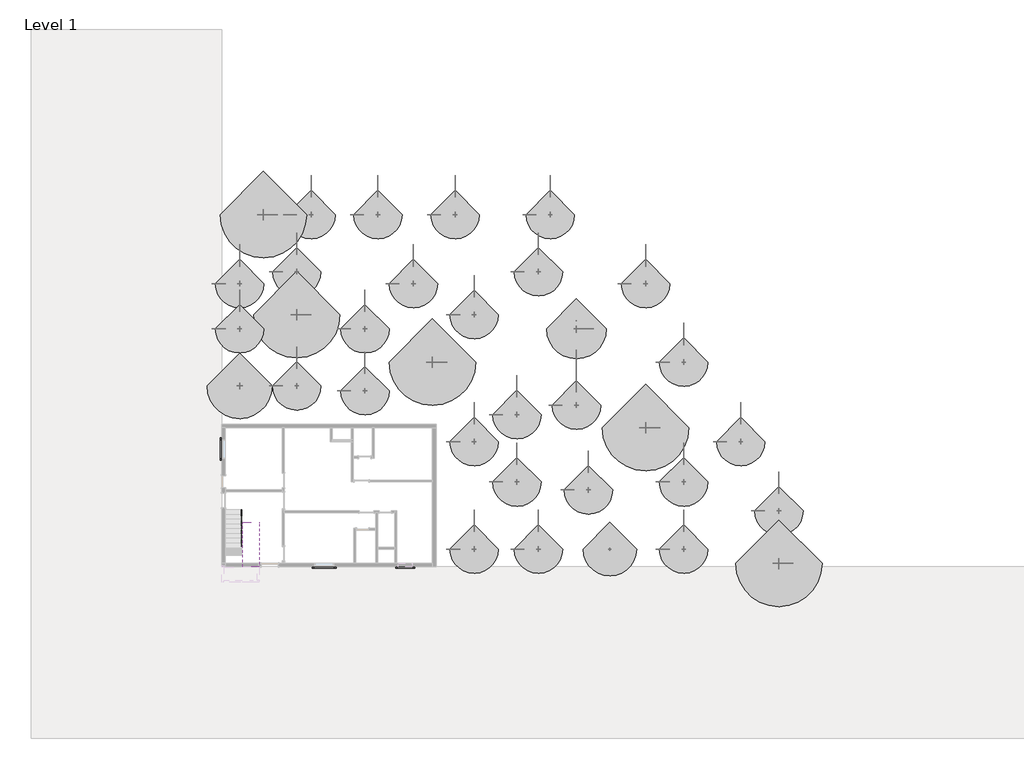
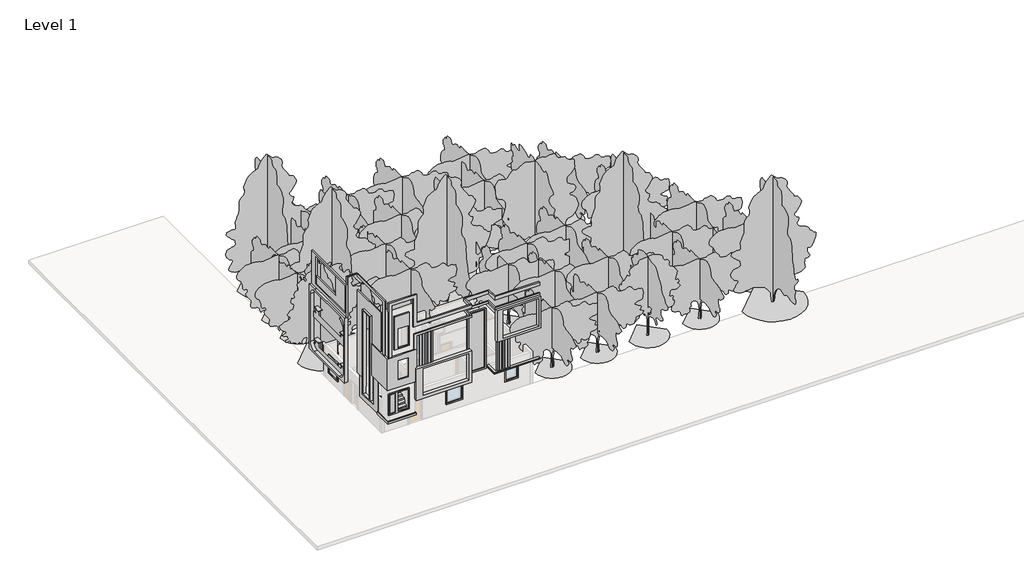
# One storey, part 2 of 2: 34 geographic elements, 1 proxy, 1 railing, 1 stair flight.
"""IFC4 building model written with IfcOpenShell, lengths in millimetres."""

from ifc_helpers import new_model, si_unit, frame, origin, place, context, project, spatial, polyline, outline, extrude, faceted_brep, transform, mapped, element, save
from components import generic_models_1_generic_models_1_784ad703, rpc_tree_deciduous_common_apple_20_2cf08d23, rpc_tree_deciduous_largetooth_aspen_25_f6cd7aa4, rpc_tree_deciduous_lombardy_poplar_40_01077960, rpc_tree_deciduous_red_maple_30_cba750cc, rpc_tree_deciduous_schumard_oak_30_cf07c7db

model = new_model("IFC4")

# Units and contexts
model_context = context("Model", 3, world=origin())
ifc_project = project(units=[si_unit("LENGTHUNIT", "METRE", prefix="MILLI")], contexts=[model_context])

# Site, building, storey
site = spatial("IfcSite", under=ifc_project)
building = spatial("IfcBuilding", under=site)
storey = spatial("IfcBuildingStorey", under=building, Name="Level 1", Elevation=0.0)

# Proxy
placement = place(None, origin())
generic_models_1_generic_models_1_shape = generic_models_1_generic_models_1_784ad703(model_context)
element("IfcBuildingElementProxy", 1, Name="Generic Models 1 : Generic Models 1", ObjectType="Generic Models 1 : Generic Models 1", at=placement, inside=storey, context=model_context, shape_type="MappedRepresentation", body=[
    mapped(generic_models_1_generic_models_1_shape, transform((0.0, 0.0, 0.0), x_axis=(1.0, 0.0, 0.0), y_axis=(0.0, 1.0, 0.0), z_axis=(0.0, 0.0, 1.0))),
])

# Geographic elements
rpc_tree_deciduous_common_apple_20_shape = rpc_tree_deciduous_common_apple_20_2cf08d23(model_context)
element("IfcGeographicElement", 2, ObjectType="RPC Tree - Deciduous : Common Apple - 20'", at=placement, inside=storey, context=model_context, shape_type="MappedRepresentation", body=[
    mapped(rpc_tree_deciduous_common_apple_20_shape, transform((-9198.7394758, 21766.0495492, 0.0), x_axis=(1.0, 0.0, 0.0), y_axis=(0.0, 1.0, 0.0), z_axis=(0.0, 0.0, 1.0))),
])
element("IfcGeographicElement", 3, ObjectType="RPC Tree - Deciduous : Common Apple - 20'", at=placement, inside=storey, context=model_context, shape_type="MappedRepresentation", body=[
    mapped(rpc_tree_deciduous_common_apple_20_shape, transform((-9198.7394758, 18870.4495492, 0.0), x_axis=(1.0, 0.0, 0.0), y_axis=(0.0, 1.0, 0.0), z_axis=(0.0, 0.0, 1.0))),
])
element("IfcGeographicElement", 4, ObjectType="RPC Tree - Deciduous : Common Apple - 20'", at=placement, inside=storey, context=model_context, shape_type="MappedRepresentation", body=[
    mapped(rpc_tree_deciduous_common_apple_20_shape, transform((-5541.1394758, 15212.8495492, 0.0), x_axis=(1.0, 0.0, 0.0), y_axis=(0.0, 1.0, 0.0), z_axis=(0.0, 0.0, 1.0))),
])
element("IfcGeographicElement", 5, ObjectType="RPC Tree - Deciduous : Common Apple - 20'", at=placement, inside=storey, context=model_context, shape_type="MappedRepresentation", body=[
    mapped(rpc_tree_deciduous_common_apple_20_shape, transform((-1172.3394758, 18870.4495492, 0.0), x_axis=(1.0, 0.0, 0.0), y_axis=(0.0, 1.0, 0.0), z_axis=(0.0, 0.0, 1.0))),
])
element("IfcGeographicElement", 6, ObjectType="RPC Tree - Deciduous : Common Apple - 20'", at=placement, inside=storey, context=model_context, shape_type="MappedRepresentation", body=[
    mapped(rpc_tree_deciduous_common_apple_20_shape, transform((-1172.3394758, 14908.0495492, 0.0), x_axis=(1.0, 0.0, 0.0), y_axis=(0.0, 1.0, 0.0), z_axis=(0.0, 0.0, 1.0))),
])
element("IfcGeographicElement", 7, ObjectType="RPC Tree - Deciduous : Common Apple - 20'", at=placement, inside=storey, context=model_context, shape_type="MappedRepresentation", body=[
    mapped(rpc_tree_deciduous_common_apple_20_shape, transform((5812.6605242, 4773.4495492, 0.0), x_axis=(1.0, 0.0, 0.0), y_axis=(0.0, 1.0, 0.0), z_axis=(0.0, 0.0, 1.0))),
])
element("IfcGeographicElement", 8, ObjectType="RPC Tree - Deciduous : Common Apple - 20'", at=placement, inside=storey, context=model_context, shape_type="MappedRepresentation", body=[
    mapped(rpc_tree_deciduous_common_apple_20_shape, transform((9927.4605242, 4773.4495492, 0.0), x_axis=(1.0, 0.0, 0.0), y_axis=(0.0, 1.0, 0.0), z_axis=(0.0, 0.0, 1.0))),
])
element("IfcGeographicElement", 9, ObjectType="RPC Tree - Deciduous : Common Apple - 20'", at=placement, inside=storey, context=model_context, shape_type="MappedRepresentation", body=[
    mapped(rpc_tree_deciduous_common_apple_20_shape, transform((13127.8605242, 8558.0495492, 0.0), x_axis=(1.0, 0.0, 0.0), y_axis=(0.0, 1.0, 0.0), z_axis=(0.0, 0.0, 1.0))),
])
element("IfcGeographicElement", 10, ObjectType="RPC Tree - Deciduous : Common Apple - 20'", at=placement, inside=storey, context=model_context, shape_type="MappedRepresentation", body=[
    mapped(rpc_tree_deciduous_common_apple_20_shape, transform((8555.8605242, 9066.0495492, 0.0), x_axis=(1.0, 0.0, 0.0), y_axis=(0.0, 1.0, 0.0), z_axis=(0.0, 0.0, 1.0))),
])
element("IfcGeographicElement", 11, ObjectType="RPC Tree - Deciduous : Common Apple - 20'", at=placement, inside=storey, context=model_context, shape_type="MappedRepresentation", body=[
    mapped(rpc_tree_deciduous_common_apple_20_shape, transform((8555.8605242, 13384.0495492, 0.0), x_axis=(1.0, 0.0, 0.0), y_axis=(0.0, 1.0, 0.0), z_axis=(0.0, 0.0, 1.0))),
])
element("IfcGeographicElement", 12, ObjectType="RPC Tree - Deciduous : Common Apple - 20'", at=placement, inside=storey, context=model_context, shape_type="MappedRepresentation", body=[
    mapped(rpc_tree_deciduous_common_apple_20_shape, transform((12365.8605242, 13993.6495492, 0.0), x_axis=(1.0, 0.0, 0.0), y_axis=(0.0, 1.0, 0.0), z_axis=(0.0, 0.0, 1.0))),
])
element("IfcGeographicElement", 13, ObjectType="RPC Tree - Deciduous : Common Apple - 20'", at=placement, inside=storey, context=model_context, shape_type="MappedRepresentation", body=[
    mapped(rpc_tree_deciduous_common_apple_20_shape, transform((5812.6605242, 11656.8495492, 0.0), x_axis=(1.0, 0.0, 0.0), y_axis=(0.0, 1.0, 0.0), z_axis=(0.0, 0.0, 1.0))),
])
element("IfcGeographicElement", 14, ObjectType="RPC Tree - Deciduous : Common Apple - 20'", at=placement, inside=storey, context=model_context, shape_type="MappedRepresentation", body=[
    mapped(rpc_tree_deciduous_common_apple_20_shape, transform((19223.8605242, 4773.4495492, 0.0), x_axis=(1.0, 0.0, 0.0), y_axis=(0.0, 1.0, 0.0), z_axis=(0.0, 0.0, 1.0))),
])
element("IfcGeographicElement", 15, ObjectType="RPC Tree - Deciduous : Common Apple - 20'", at=placement, inside=storey, context=model_context, shape_type="MappedRepresentation", body=[
    mapped(rpc_tree_deciduous_common_apple_20_shape, transform((19223.8605242, 9066.0495492, 0.0), x_axis=(1.0, 0.0, 0.0), y_axis=(0.0, 1.0, 0.0), z_axis=(0.0, 0.0, 1.0))),
])
element("IfcGeographicElement", 16, ObjectType="RPC Tree - Deciduous : Common Apple - 20'", at=placement, inside=storey, context=model_context, shape_type="MappedRepresentation", body=[
    mapped(rpc_tree_deciduous_common_apple_20_shape, transform((5812.6605242, 19784.8495492, 0.0), x_axis=(1.0, 0.0, 0.0), y_axis=(0.0, 1.0, 0.0), z_axis=(0.0, 0.0, 1.0))),
])
element("IfcGeographicElement", 17, ObjectType="RPC Tree - Deciduous : Common Apple - 20'", at=placement, inside=storey, context=model_context, shape_type="MappedRepresentation", body=[
    mapped(rpc_tree_deciduous_common_apple_20_shape, transform((1926.4605242, 21766.0495492, 0.0), x_axis=(1.0, 0.0, 0.0), y_axis=(0.0, 1.0, 0.0), z_axis=(0.0, 0.0, 1.0))),
])
element("IfcGeographicElement", 18, ObjectType="RPC Tree - Deciduous : Common Apple - 20'", at=placement, inside=storey, context=model_context, shape_type="MappedRepresentation", body=[
    mapped(rpc_tree_deciduous_common_apple_20_shape, transform((9927.4605242, 22528.0495492, 0.0), x_axis=(1.0, 0.0, 0.0), y_axis=(0.0, 1.0, 0.0), z_axis=(0.0, 0.0, 1.0))),
])
element("IfcGeographicElement", 19, ObjectType="RPC Tree - Deciduous : Common Apple - 20'", at=placement, inside=storey, context=model_context, shape_type="MappedRepresentation", body=[
    mapped(rpc_tree_deciduous_common_apple_20_shape, transform((16785.4605242, 21766.0495492, 0.0), x_axis=(1.0, 0.0, 0.0), y_axis=(0.0, 1.0, 0.0), z_axis=(0.0, 0.0, 1.0))),
])
element("IfcGeographicElement", 20, ObjectType="RPC Tree - Deciduous : Common Apple - 20'", at=placement, inside=storey, context=model_context, shape_type="MappedRepresentation", body=[
    mapped(rpc_tree_deciduous_common_apple_20_shape, transform((19223.8605242, 16736.8495492, 0.0), x_axis=(1.0, 0.0, 0.0), y_axis=(0.0, 1.0, 0.0), z_axis=(0.0, 0.0, 1.0))),
])
element("IfcGeographicElement", 21, ObjectType="RPC Tree - Deciduous : Common Apple - 20'", at=placement, inside=storey, context=model_context, shape_type="MappedRepresentation", body=[
    mapped(rpc_tree_deciduous_common_apple_20_shape, transform((22881.4605242, 11656.8495492, 0.0), x_axis=(1.0, 0.0, 0.0), y_axis=(0.0, 1.0, 0.0), z_axis=(0.0, 0.0, 1.0))),
])
element("IfcGeographicElement", 22, ObjectType="RPC Tree - Deciduous : Common Apple - 20'", at=placement, inside=storey, context=model_context, shape_type="MappedRepresentation", body=[
    mapped(rpc_tree_deciduous_common_apple_20_shape, transform((25319.8605242, 7211.8495492, 0.0), x_axis=(1.0, 0.0, 0.0), y_axis=(0.0, 1.0, 0.0), z_axis=(0.0, 0.0, 1.0))),
])
element("IfcGeographicElement", 23, ObjectType="RPC Tree - Deciduous : Common Apple - 20'", at=placement, inside=storey, context=model_context, shape_type="MappedRepresentation", body=[
    mapped(rpc_tree_deciduous_common_apple_20_shape, transform((-4626.7394758, 26185.6495492, 0.0), x_axis=(1.0, 0.0, 0.0), y_axis=(0.0, 1.0, 0.0), z_axis=(0.0, 0.0, 1.0))),
])
element("IfcGeographicElement", 24, ObjectType="RPC Tree - Deciduous : Common Apple - 20'", at=placement, inside=storey, context=model_context, shape_type="MappedRepresentation", body=[
    mapped(rpc_tree_deciduous_common_apple_20_shape, transform((-346.8394758, 26185.6495492, 0.0), x_axis=(1.0, 0.0, 0.0), y_axis=(0.0, 1.0, 0.0), z_axis=(0.0, 0.0, 1.0))),
])
element("IfcGeographicElement", 25, ObjectType="RPC Tree - Deciduous : Common Apple - 20'", at=placement, inside=storey, context=model_context, shape_type="MappedRepresentation", body=[
    mapped(rpc_tree_deciduous_common_apple_20_shape, transform((-5541.1394758, 22528.0495492, 0.0), x_axis=(1.0, 0.0, 0.0), y_axis=(0.0, 1.0, 0.0), z_axis=(0.0, 0.0, 1.0))),
])
element("IfcGeographicElement", 26, ObjectType="RPC Tree - Deciduous : Common Apple - 20'", at=placement, inside=storey, context=model_context, shape_type="MappedRepresentation", body=[
    mapped(rpc_tree_deciduous_common_apple_20_shape, transform((4593.4605242, 26185.6495492, 0.0), x_axis=(1.0, 0.0, 0.0), y_axis=(0.0, 1.0, 0.0), z_axis=(0.0, 0.0, 1.0))),
])
element("IfcGeographicElement", 27, ObjectType="RPC Tree - Deciduous : Common Apple - 20'", at=placement, inside=storey, context=model_context, shape_type="MappedRepresentation", body=[
    mapped(rpc_tree_deciduous_common_apple_20_shape, transform((10689.4605242, 26185.6495492, 0.0), x_axis=(1.0, 0.0, 0.0), y_axis=(0.0, 1.0, 0.0), z_axis=(0.0, 0.0, 1.0))),
])
rpc_tree_deciduous_largetooth_aspen_25_shape = rpc_tree_deciduous_largetooth_aspen_25_f6cd7aa4(model_context)
element("IfcGeographicElement", 28, ObjectType="RPC Tree - Deciduous : Largetooth Aspen - 25'", at=placement, inside=storey, context=model_context, shape_type="MappedRepresentation", body=[
    mapped(rpc_tree_deciduous_largetooth_aspen_25_shape, transform((14499.4605242, 4773.4495492, 0.0), x_axis=(1.0, 0.0, 0.0), y_axis=(0.0, 1.0, 0.0), z_axis=(0.0, 0.0, 1.0))),
])
rpc_tree_deciduous_lombardy_poplar_40_shape = rpc_tree_deciduous_lombardy_poplar_40_01077960(model_context)
element("IfcGeographicElement", 29, ObjectType="RPC Tree - Deciduous : Lombardy Poplar - 40'", at=placement, inside=storey, context=model_context, shape_type="MappedRepresentation", body=[
    mapped(rpc_tree_deciduous_lombardy_poplar_40_shape, transform((-5541.1394758, 19784.8495492, 0.0), x_axis=(1.0, 0.0, 0.0), y_axis=(0.0, 1.0, 0.0), z_axis=(0.0, 0.0, 1.0))),
])
element("IfcGeographicElement", 30, ObjectType="RPC Tree - Deciduous : Lombardy Poplar - 40'", at=placement, inside=storey, context=model_context, shape_type="MappedRepresentation", body=[
    mapped(rpc_tree_deciduous_lombardy_poplar_40_shape, transform((3145.6605242, 16736.8495492, 0.0), x_axis=(1.0, 0.0, 0.0), y_axis=(0.0, 1.0, 0.0), z_axis=(0.0, 0.0, 1.0))),
])
element("IfcGeographicElement", 31, ObjectType="RPC Tree - Deciduous : Lombardy Poplar - 40'", at=placement, inside=storey, context=model_context, shape_type="MappedRepresentation", body=[
    mapped(rpc_tree_deciduous_lombardy_poplar_40_shape, transform((16785.4605242, 12545.8495492, 0.0), x_axis=(1.0, 0.0, 0.0), y_axis=(0.0, 1.0, 0.0), z_axis=(0.0, 0.0, 1.0))),
])
element("IfcGeographicElement", 32, ObjectType="RPC Tree - Deciduous : Lombardy Poplar - 40'", at=placement, inside=storey, context=model_context, shape_type="MappedRepresentation", body=[
    mapped(rpc_tree_deciduous_lombardy_poplar_40_shape, transform((25319.8605242, 3859.0495492, 0.0), x_axis=(1.0, 0.0, 0.0), y_axis=(0.0, 1.0, 0.0), z_axis=(0.0, 0.0, 1.0))),
])
element("IfcGeographicElement", 33, ObjectType="RPC Tree - Deciduous : Lombardy Poplar - 40'", at=placement, inside=storey, context=model_context, shape_type="MappedRepresentation", body=[
    mapped(rpc_tree_deciduous_lombardy_poplar_40_shape, transform((-7674.7394758, 26185.6495492, 0.0), x_axis=(1.0, 0.0, 0.0), y_axis=(0.0, 1.0, 0.0), z_axis=(0.0, 0.0, 1.0))),
])
rpc_tree_deciduous_red_maple_30_shape = rpc_tree_deciduous_red_maple_30_cba750cc(model_context)
element("IfcGeographicElement", 34, ObjectType="RPC Tree - Deciduous : Red Maple - 30'", at=placement, inside=storey, context=model_context, shape_type="MappedRepresentation", body=[
    mapped(rpc_tree_deciduous_red_maple_30_shape, transform((-9198.7394758, 15212.8495492, 0.0), x_axis=(1.0, 0.0, 0.0), y_axis=(0.0, 1.0, 0.0), z_axis=(0.0, 0.0, 1.0))),
])
rpc_tree_deciduous_schumard_oak_30_shape = rpc_tree_deciduous_schumard_oak_30_cf07c7db(model_context)
element("IfcGeographicElement", 35, ObjectType="RPC Tree - Deciduous : Schumard Oak - 30'", at=placement, inside=storey, context=model_context, shape_type="MappedRepresentation", body=[
    mapped(rpc_tree_deciduous_schumard_oak_30_shape, transform((12365.8605242, 18870.4495492, 0.0), x_axis=(1.0, 0.0, 0.0), y_axis=(0.0, 1.0, 0.0), z_axis=(0.0, 0.0, 1.0))),
])

# Railing
element("IfcRailing", 36, ObjectType="Handrail - Rectangular", at=placement, inside=storey, context=model_context, shape_type="SolidModel", body=[
    faceted_brep([(-9046.3394758, 7288.0495492, 1059.5428571), (-9046.3394758, 7288.0495492, 1003.2772447), (-9097.1394758, 7288.0495492, 1003.2772447), (-9097.1394758, 7288.0495492, 1059.5428571), (-9046.3394758, 3935.2495492, 2656.1142857), (-9046.3394758, 3923.7717632, 2605.3142857), (-9097.1394758, 3923.7717632, 2605.3142857), (-9097.1394758, 3935.2495492, 2656.1142857), (-9046.3394758, 3630.4495492, 2656.1142857), (-9097.1394758, 3630.4495492, 2656.1142857), (-9097.1394758, 3579.6495492, 2605.3142857), (-9046.3394758, 3579.6495492, 2605.3142857)], [[[0, 1, 2, 3]], [[1, 0, 4, 5]], [[2, 1, 5, 6]], [[3, 2, 6, 7]], [[0, 3, 7, 4]], [[8, 9, 10, 11]], [[5, 4, 8, 11]], [[6, 5, 11, 10]], [[7, 6, 10, 9]], [[4, 7, 9, 8]]]),
    faceted_brep([(-9046.3394758, 3630.4495492, 2656.1142857), (-9046.3394758, 3579.6495492, 2605.3142857), (-9097.1394758, 3579.6495492, 2605.3142857), (-9097.1394758, 3630.4495492, 2656.1142857), (-9046.3394758, 3630.4495492, 2786.7428571), (-9097.1394758, 3630.4495492, 2837.5428571), (-9097.1394758, 3579.6495492, 2837.5428571), (-9046.3394758, 3579.6495492, 2786.7428571)], [[[0, 1, 2, 3]], [[4, 5, 6, 7]], [[1, 0, 4, 7]], [[2, 1, 7, 6]], [[3, 2, 6, 5]], [[0, 3, 5, 4]]]),
    faceted_brep([(-9097.1394758, 3630.4495492, 2837.5428571), (-9046.3394758, 3630.4495492, 2786.7428571), (-9046.3394758, 3579.6495492, 2786.7428571), (-9097.1394758, 3579.6495492, 2837.5428571), (-8995.5394758, 3630.4495492, 2837.5428571), (-8995.5394758, 3630.4495492, 2786.7428571), (-8944.7394758, 3579.6495492, 2786.7428571), (-8944.7394758, 3579.6495492, 2837.5428571), (-8995.5394758, 3706.6495492, 2837.5428571), (-8995.5394758, 3718.1273353, 2786.7428571), (-8944.7394758, 3718.1273353, 2786.7428571), (-8944.7394758, 3706.6495492, 2837.5428571), (-8995.5394758, 6068.8495492, 3962.4), (-8995.5394758, 6080.3273353, 3911.6), (-8944.7394758, 6080.3273353, 3911.6), (-8944.7394758, 6068.8495492, 3962.4), (-8995.5394758, 6373.6495492, 3962.4), (-8944.7394758, 6373.6495492, 3962.4), (-8944.7394758, 6373.6495492, 3911.6), (-8995.5394758, 6373.6495492, 3911.6)], [[[0, 1, 2, 3]], [[1, 0, 4, 5]], [[2, 1, 5, 6]], [[3, 2, 6, 7]], [[0, 3, 7, 4]], [[5, 4, 8, 9]], [[6, 5, 9, 10]], [[7, 6, 10, 11]], [[4, 7, 11, 8]], [[9, 8, 12, 13]], [[10, 9, 13, 14]], [[11, 10, 14, 15]], [[8, 11, 15, 12]], [[16, 17, 18, 19]], [[13, 12, 16, 19]], [[14, 13, 19, 18]], [[15, 14, 18, 17]], [[12, 15, 17, 16]]]),
    extrude(outline(polyline([(-8979.6644758, 6338.7245492), (-8979.6644758, 6357.7745492), (-8960.6144758, 6357.7745492), (-8960.6144758, 6338.7245492), (-8979.6644758, 6338.7245492)])), frame((0.0, 0.0, 3048.0), z_axis=(0.0, 0.0, 1.0), x_axis=(1.0, 0.0, 0.0)), (0.0, 0.0, 1.0), 863.6),
    extrude(outline(polyline([(-8979.6644758, 6237.1245492), (-8979.6644758, 6256.1745492), (-8960.6144758, 6256.1745492), (-8960.6144758, 6237.1245492), (-8979.6644758, 6237.1245492)])), frame((0.0, 0.0, 3048.0), z_axis=(0.0, 0.0, 1.0), x_axis=(1.0, 0.0, 0.0)), (0.0, 0.0, 1.0), 863.6),
    extrude(outline(polyline([(-8979.6644758, 6135.5245492), (-8979.6644758, 6154.5745492), (-8960.6144758, 6154.5745492), (-8960.6144758, 6135.5245492), (-8979.6644758, 6135.5245492)])), frame((0.0, 0.0, 3048.0), z_axis=(0.0, 0.0, 1.0), x_axis=(1.0, 0.0, 0.0)), (0.0, 0.0, 1.0), 863.6),
    extrude(outline(polyline([(6052.9745492, 3898.5748638), (6052.9745492, 2902.8571429), (6033.9245492, 2902.8571429), (6033.9245492, 3889.5034352), (6052.9745492, 3898.5748638)])), frame((-8979.6644758, 0.0, 0.0), z_axis=(1.0, 0.0, 0.0), x_axis=(0.0, 1.0, 0.0)), (0.0, 0.0, 1.0), 19.05),
    extrude(outline(polyline([(5951.3745492, 3850.1939114), (5951.3745492, 2902.8571429), (5932.3245492, 2902.8571429), (5932.3245492, 3841.1224828), (5951.3745492, 3850.1939114)])), frame((-8979.6644758, 0.0, 0.0), z_axis=(1.0, 0.0, 0.0), x_axis=(0.0, 1.0, 0.0)), (0.0, 0.0, 1.0), 19.05),
    extrude(outline(polyline([(5849.7745492, 3801.812959), (5849.7745492, 2902.8571429), (5830.7245492, 2902.8571429), (5830.7245492, 3792.7415305), (5849.7745492, 3801.812959)])), frame((-8979.6644758, 0.0, 0.0), z_axis=(1.0, 0.0, 0.0), x_axis=(0.0, 1.0, 0.0)), (0.0, 0.0, 1.0), 19.05),
    extrude(outline(polyline([(5748.1745492, 3753.4320067), (5748.1745492, 2757.7142857), (5729.1245492, 2757.7142857), (5729.1245492, 3744.3605781), (5748.1745492, 3753.4320067)])), frame((-8979.6644758, 0.0, 0.0), z_axis=(1.0, 0.0, 0.0), x_axis=(0.0, 1.0, 0.0)), (0.0, 0.0, 1.0), 19.05),
    extrude(outline(polyline([(5646.5745492, 3705.0510543), (5646.5745492, 2757.7142857), (5627.5245492, 2757.7142857), (5627.5245492, 3695.9796257), (5646.5745492, 3705.0510543)])), frame((-8979.6644758, 0.0, 0.0), z_axis=(1.0, 0.0, 0.0), x_axis=(0.0, 1.0, 0.0)), (0.0, 0.0, 1.0), 19.05),
    extrude(outline(polyline([(5544.9745492, 3656.6701019), (5544.9745492, 2757.7142857), (5525.9245492, 2757.7142857), (5525.9245492, 3647.5986733), (5544.9745492, 3656.6701019)])), frame((-8979.6644758, 0.0, 0.0), z_axis=(1.0, 0.0, 0.0), x_axis=(0.0, 1.0, 0.0)), (0.0, 0.0, 1.0), 19.05),
    extrude(outline(polyline([(5443.3745492, 3608.2891495), (5443.3745492, 2612.5714286), (5424.3245492, 2612.5714286), (5424.3245492, 3599.2177209), (5443.3745492, 3608.2891495)])), frame((-8979.6644758, 0.0, 0.0), z_axis=(1.0, 0.0, 0.0), x_axis=(0.0, 1.0, 0.0)), (0.0, 0.0, 1.0), 19.05),
    extrude(outline(polyline([(5341.7745492, 3559.9081971), (5341.7745492, 2612.5714286), (5322.7245492, 2612.5714286), (5322.7245492, 3550.8367686), (5341.7745492, 3559.9081971)])), frame((-8979.6644758, 0.0, 0.0), z_axis=(1.0, 0.0, 0.0), x_axis=(0.0, 1.0, 0.0)), (0.0, 0.0, 1.0), 19.05),
    extrude(outline(polyline([(5240.1745492, 3511.5272447), (5240.1745492, 2612.5714286), (5221.1245492, 2612.5714286), (5221.1245492, 3502.4558162), (5240.1745492, 3511.5272447)])), frame((-8979.6644758, 0.0, 0.0), z_axis=(1.0, 0.0, 0.0), x_axis=(0.0, 1.0, 0.0)), (0.0, 0.0, 1.0), 19.05),
    extrude(outline(polyline([(5138.5745492, 3463.1462924), (5138.5745492, 2467.4285714), (5119.5245492, 2467.4285714), (5119.5245492, 3454.0748638), (5138.5745492, 3463.1462924)])), frame((-8979.6644758, 0.0, 0.0), z_axis=(1.0, 0.0, 0.0), x_axis=(0.0, 1.0, 0.0)), (0.0, 0.0, 1.0), 19.05),
    extrude(outline(polyline([(5036.9745492, 3414.76534), (5036.9745492, 2467.4285714), (5017.9245492, 2467.4285714), (5017.9245492, 3405.6939114), (5036.9745492, 3414.76534)])), frame((-8979.6644758, 0.0, 0.0), z_axis=(1.0, 0.0, 0.0), x_axis=(0.0, 1.0, 0.0)), (0.0, 0.0, 1.0), 19.05),
    extrude(outline(polyline([(4935.3745492, 3366.3843876), (4935.3745492, 2467.4285714), (4916.3245492, 2467.4285714), (4916.3245492, 3357.312959), (4935.3745492, 3366.3843876)])), frame((-8979.6644758, 0.0, 0.0), z_axis=(1.0, 0.0, 0.0), x_axis=(0.0, 1.0, 0.0)), (0.0, 0.0, 1.0), 19.05),
    extrude(outline(polyline([(4833.7745492, 3318.0034352), (4833.7745492, 2322.2857143), (4814.7245492, 2322.2857143), (4814.7245492, 3308.9320067), (4833.7745492, 3318.0034352)])), frame((-8979.6644758, 0.0, 0.0), z_axis=(1.0, 0.0, 0.0), x_axis=(0.0, 1.0, 0.0)), (0.0, 0.0, 1.0), 19.05),
    extrude(outline(polyline([(4732.1745492, 3269.6224828), (4732.1745492, 2322.2857143), (4713.1245492, 2322.2857143), (4713.1245492, 3260.5510543), (4732.1745492, 3269.6224828)])), frame((-8979.6644758, 0.0, 0.0), z_axis=(1.0, 0.0, 0.0), x_axis=(0.0, 1.0, 0.0)), (0.0, 0.0, 1.0), 19.05),
    extrude(outline(polyline([(4630.5745492, 3221.2415305), (4630.5745492, 2322.2857143), (4611.5245492, 2322.2857143), (4611.5245492, 3212.1701019), (4630.5745492, 3221.2415305)])), frame((-8979.6644758, 0.0, 0.0), z_axis=(1.0, 0.0, 0.0), x_axis=(0.0, 1.0, 0.0)), (0.0, 0.0, 1.0), 19.05),
    extrude(outline(polyline([(4528.9745492, 3172.8605781), (4528.9745492, 2177.1428571), (4509.9245492, 2177.1428571), (4509.9245492, 3163.7891495), (4528.9745492, 3172.8605781)])), frame((-8979.6644758, 0.0, 0.0), z_axis=(1.0, 0.0, 0.0), x_axis=(0.0, 1.0, 0.0)), (0.0, 0.0, 1.0), 19.05),
    extrude(outline(polyline([(4427.3745492, 3124.4796257), (4427.3745492, 2177.1428571), (4408.3245492, 2177.1428571), (4408.3245492, 3115.4081971), (4427.3745492, 3124.4796257)])), frame((-8979.6644758, 0.0, 0.0), z_axis=(1.0, 0.0, 0.0), x_axis=(0.0, 1.0, 0.0)), (0.0, 0.0, 1.0), 19.05),
    extrude(outline(polyline([(4325.7745492, 3076.0986733), (4325.7745492, 2177.1428571), (4306.7245492, 2177.1428571), (4306.7245492, 3067.0272447), (4325.7745492, 3076.0986733)])), frame((-8979.6644758, 0.0, 0.0), z_axis=(1.0, 0.0, 0.0), x_axis=(0.0, 1.0, 0.0)), (0.0, 0.0, 1.0), 19.05),
    extrude(outline(polyline([(4224.1745492, 3027.7177209), (4224.1745492, 2032.0), (4205.1245492, 2032.0), (4205.1245492, 3018.6462924), (4224.1745492, 3027.7177209)])), frame((-8979.6644758, 0.0, 0.0), z_axis=(1.0, 0.0, 0.0), x_axis=(0.0, 1.0, 0.0)), (0.0, 0.0, 1.0), 19.05),
    extrude(outline(polyline([(4122.5745492, 2979.3367686), (4122.5745492, 2032.0), (4103.5245492, 2032.0), (4103.5245492, 2970.26534), (4122.5745492, 2979.3367686)])), frame((-8979.6644758, 0.0, 0.0), z_axis=(1.0, 0.0, 0.0), x_axis=(0.0, 1.0, 0.0)), (0.0, 0.0, 1.0), 19.05),
    extrude(outline(polyline([(4020.9745492, 2930.9558162), (4020.9745492, 2032.0), (4001.9245492, 2032.0), (4001.9245492, 2921.8843876), (4020.9745492, 2930.9558162)])), frame((-8979.6644758, 0.0, 0.0), z_axis=(1.0, 0.0, 0.0), x_axis=(0.0, 1.0, 0.0)), (0.0, 0.0, 1.0), 19.05),
    extrude(outline(polyline([(3919.3745492, 2882.5748638), (3919.3745492, 1886.8571429), (3900.3245492, 1886.8571429), (3900.3245492, 2873.5034352), (3919.3745492, 2882.5748638)])), frame((-8979.6644758, 0.0, 0.0), z_axis=(1.0, 0.0, 0.0), x_axis=(0.0, 1.0, 0.0)), (0.0, 0.0, 1.0), 19.05),
    extrude(outline(polyline([(3817.7745492, 2834.1939114), (3817.7745492, 1886.8571429), (3798.7245492, 1886.8571429), (3798.7245492, 2825.1224828), (3817.7745492, 2834.1939114)])), frame((-8979.6644758, 0.0, 0.0), z_axis=(1.0, 0.0, 0.0), x_axis=(0.0, 1.0, 0.0)), (0.0, 0.0, 1.0), 19.05),
    extrude(outline(polyline([(3716.1745492, 2785.812959), (3716.1745492, 1886.8571429), (3697.1245492, 1886.8571429), (3697.1245492, 2776.7415305), (3716.1745492, 2785.812959)])), frame((-8979.6644758, 0.0, 0.0), z_axis=(1.0, 0.0, 0.0), x_axis=(0.0, 1.0, 0.0)), (0.0, 0.0, 1.0), 19.05),
    extrude(outline(polyline([(-9062.2144758, 3639.9745492), (-9062.2144758, 3620.9245492), (-9081.2644758, 3620.9245492), (-9081.2644758, 3639.9745492), (-9062.2144758, 3639.9745492)])), frame((0.0, 0.0, 1741.7142857), z_axis=(0.0, 0.0, 1.0), x_axis=(1.0, 0.0, 0.0)), (0.0, 0.0, 1.0), 863.6),
    extrude(outline(polyline([(-9062.2144758, 3741.5745492), (-9062.2144758, 3722.5245492), (-9081.2644758, 3722.5245492), (-9081.2644758, 3741.5745492), (-9062.2144758, 3741.5745492)])), frame((0.0, 0.0, 1741.7142857), z_axis=(0.0, 0.0, 1.0), x_axis=(1.0, 0.0, 0.0)), (0.0, 0.0, 1.0), 863.6),
    extrude(outline(polyline([(-9062.2144758, 3843.1745492), (-9062.2144758, 3824.1245492), (-9081.2644758, 3824.1245492), (-9081.2644758, 3843.1745492), (-9062.2144758, 3843.1745492)])), frame((0.0, 0.0, 1741.7142857), z_axis=(0.0, 0.0, 1.0), x_axis=(1.0, 0.0, 0.0)), (0.0, 0.0, 1.0), 863.6),
    extrude(outline(polyline([(3944.7745492, 2595.312959), (3944.7745492, 1741.7142857), (3925.7245492, 1741.7142857), (3925.7245492, 2604.3843876), (3944.7745492, 2595.312959)])), frame((-9081.2644758, 0.0, 0.0), z_axis=(1.0, 0.0, 0.0), x_axis=(0.0, 1.0, 0.0)), (0.0, 0.0, 1.0), 19.05),
    extrude(outline(polyline([(4046.3745492, 2546.9320067), (4046.3745492, 1596.5714286), (4027.3245492, 1596.5714286), (4027.3245492, 2556.0034352), (4046.3745492, 2546.9320067)])), frame((-9081.2644758, 0.0, 0.0), z_axis=(1.0, 0.0, 0.0), x_axis=(0.0, 1.0, 0.0)), (0.0, 0.0, 1.0), 19.05),
    extrude(outline(polyline([(4147.9745492, 2498.5510543), (4147.9745492, 1596.5714286), (4128.9245492, 1596.5714286), (4128.9245492, 2507.6224828), (4147.9745492, 2498.5510543)])), frame((-9081.2644758, 0.0, 0.0), z_axis=(1.0, 0.0, 0.0), x_axis=(0.0, 1.0, 0.0)), (0.0, 0.0, 1.0), 19.05),
    extrude(outline(polyline([(4249.5745492, 2450.1701019), (4249.5745492, 1596.5714286), (4230.5245492, 1596.5714286), (4230.5245492, 2459.2415305), (4249.5745492, 2450.1701019)])), frame((-9081.2644758, 0.0, 0.0), z_axis=(1.0, 0.0, 0.0), x_axis=(0.0, 1.0, 0.0)), (0.0, 0.0, 1.0), 19.05),
    extrude(outline(polyline([(4351.1745492, 2401.7891495), (4351.1745492, 1451.4285714), (4332.1245492, 1451.4285714), (4332.1245492, 2410.8605781), (4351.1745492, 2401.7891495)])), frame((-9081.2644758, 0.0, 0.0), z_axis=(1.0, 0.0, 0.0), x_axis=(0.0, 1.0, 0.0)), (0.0, 0.0, 1.0), 19.05),
    extrude(outline(polyline([(4452.7745492, 2353.4081971), (4452.7745492, 1451.4285714), (4433.7245492, 1451.4285714), (4433.7245492, 2362.4796257), (4452.7745492, 2353.4081971)])), frame((-9081.2644758, 0.0, 0.0), z_axis=(1.0, 0.0, 0.0), x_axis=(0.0, 1.0, 0.0)), (0.0, 0.0, 1.0), 19.05),
    extrude(outline(polyline([(4554.3745492, 2305.0272447), (4554.3745492, 1451.4285714), (4535.3245492, 1451.4285714), (4535.3245492, 2314.0986733), (4554.3745492, 2305.0272447)])), frame((-9081.2644758, 0.0, 0.0), z_axis=(1.0, 0.0, 0.0), x_axis=(0.0, 1.0, 0.0)), (0.0, 0.0, 1.0), 19.05),
    extrude(outline(polyline([(4655.9745492, 2256.6462924), (4655.9745492, 1306.2857143), (4636.9245492, 1306.2857143), (4636.9245492, 2265.7177209), (4655.9745492, 2256.6462924)])), frame((-9081.2644758, 0.0, 0.0), z_axis=(1.0, 0.0, 0.0), x_axis=(0.0, 1.0, 0.0)), (0.0, 0.0, 1.0), 19.05),
    extrude(outline(polyline([(4757.5745492, 2208.26534), (4757.5745492, 1306.2857143), (4738.5245492, 1306.2857143), (4738.5245492, 2217.3367686), (4757.5745492, 2208.26534)])), frame((-9081.2644758, 0.0, 0.0), z_axis=(1.0, 0.0, 0.0), x_axis=(0.0, 1.0, 0.0)), (0.0, 0.0, 1.0), 19.05),
    extrude(outline(polyline([(4859.1745492, 2159.8843876), (4859.1745492, 1306.2857143), (4840.1245492, 1306.2857143), (4840.1245492, 2168.9558162), (4859.1745492, 2159.8843876)])), frame((-9081.2644758, 0.0, 0.0), z_axis=(1.0, 0.0, 0.0), x_axis=(0.0, 1.0, 0.0)), (0.0, 0.0, 1.0), 19.05),
    extrude(outline(polyline([(4960.7745492, 2111.5034352), (4960.7745492, 1161.1428571), (4941.7245492, 1161.1428571), (4941.7245492, 2120.5748638), (4960.7745492, 2111.5034352)])), frame((-9081.2644758, 0.0, 0.0), z_axis=(1.0, 0.0, 0.0), x_axis=(0.0, 1.0, 0.0)), (0.0, 0.0, 1.0), 19.05),
    extrude(outline(polyline([(5062.3745492, 2063.1224828), (5062.3745492, 1161.1428571), (5043.3245492, 1161.1428571), (5043.3245492, 2072.1939114), (5062.3745492, 2063.1224828)])), frame((-9081.2644758, 0.0, 0.0), z_axis=(1.0, 0.0, 0.0), x_axis=(0.0, 1.0, 0.0)), (0.0, 0.0, 1.0), 19.05),
    extrude(outline(polyline([(5163.9745492, 2014.7415305), (5163.9745492, 1161.1428571), (5144.9245492, 1161.1428571), (5144.9245492, 2023.812959), (5163.9745492, 2014.7415305)])), frame((-9081.2644758, 0.0, 0.0), z_axis=(1.0, 0.0, 0.0), x_axis=(0.0, 1.0, 0.0)), (0.0, 0.0, 1.0), 19.05),
    extrude(outline(polyline([(5265.5745492, 1966.3605781), (5265.5745492, 1016.0), (5246.5245492, 1016.0), (5246.5245492, 1975.4320067), (5265.5745492, 1966.3605781)])), frame((-9081.2644758, 0.0, 0.0), z_axis=(1.0, 0.0, 0.0), x_axis=(0.0, 1.0, 0.0)), (0.0, 0.0, 1.0), 19.05),
    extrude(outline(polyline([(5367.1745492, 1917.9796257), (5367.1745492, 1016.0), (5348.1245492, 1016.0), (5348.1245492, 1927.0510543), (5367.1745492, 1917.9796257)])), frame((-9081.2644758, 0.0, 0.0), z_axis=(1.0, 0.0, 0.0), x_axis=(0.0, 1.0, 0.0)), (0.0, 0.0, 1.0), 19.05),
    extrude(outline(polyline([(5468.7745492, 1869.5986733), (5468.7745492, 1016.0), (5449.7245492, 1016.0), (5449.7245492, 1878.6701019), (5468.7745492, 1869.5986733)])), frame((-9081.2644758, 0.0, 0.0), z_axis=(1.0, 0.0, 0.0), x_axis=(0.0, 1.0, 0.0)), (0.0, 0.0, 1.0), 19.05),
    extrude(outline(polyline([(5570.3745492, 1821.2177209), (5570.3745492, 870.8571429), (5551.3245492, 870.8571429), (5551.3245492, 1830.2891495), (5570.3745492, 1821.2177209)])), frame((-9081.2644758, 0.0, 0.0), z_axis=(1.0, 0.0, 0.0), x_axis=(0.0, 1.0, 0.0)), (0.0, 0.0, 1.0), 19.05),
    extrude(outline(polyline([(5671.9745492, 1772.8367686), (5671.9745492, 870.8571429), (5652.9245492, 870.8571429), (5652.9245492, 1781.9081971), (5671.9745492, 1772.8367686)])), frame((-9081.2644758, 0.0, 0.0), z_axis=(1.0, 0.0, 0.0), x_axis=(0.0, 1.0, 0.0)), (0.0, 0.0, 1.0), 19.05),
    extrude(outline(polyline([(5773.5745492, 1724.4558162), (5773.5745492, 870.8571429), (5754.5245492, 870.8571429), (5754.5245492, 1733.5272447), (5773.5745492, 1724.4558162)])), frame((-9081.2644758, 0.0, 0.0), z_axis=(1.0, 0.0, 0.0), x_axis=(0.0, 1.0, 0.0)), (0.0, 0.0, 1.0), 19.05),
    extrude(outline(polyline([(5875.1745492, 1676.0748638), (5875.1745492, 725.7142857), (5856.1245492, 725.7142857), (5856.1245492, 1685.1462924), (5875.1745492, 1676.0748638)])), frame((-9081.2644758, 0.0, 0.0), z_axis=(1.0, 0.0, 0.0), x_axis=(0.0, 1.0, 0.0)), (0.0, 0.0, 1.0), 19.05),
    extrude(outline(polyline([(5976.7745492, 1627.6939114), (5976.7745492, 725.7142857), (5957.7245492, 725.7142857), (5957.7245492, 1636.76534), (5976.7745492, 1627.6939114)])), frame((-9081.2644758, 0.0, 0.0), z_axis=(1.0, 0.0, 0.0), x_axis=(0.0, 1.0, 0.0)), (0.0, 0.0, 1.0), 19.05),
    extrude(outline(polyline([(6078.3745492, 1579.312959), (6078.3745492, 725.7142857), (6059.3245492, 725.7142857), (6059.3245492, 1588.3843876), (6078.3745492, 1579.312959)])), frame((-9081.2644758, 0.0, 0.0), z_axis=(1.0, 0.0, 0.0), x_axis=(0.0, 1.0, 0.0)), (0.0, 0.0, 1.0), 19.05),
    extrude(outline(polyline([(6179.9745492, 1530.9320067), (6179.9745492, 580.5714286), (6160.9245492, 580.5714286), (6160.9245492, 1540.0034352), (6179.9745492, 1530.9320067)])), frame((-9081.2644758, 0.0, 0.0), z_axis=(1.0, 0.0, 0.0), x_axis=(0.0, 1.0, 0.0)), (0.0, 0.0, 1.0), 19.05),
    extrude(outline(polyline([(6281.5745492, 1482.5510543), (6281.5745492, 580.5714286), (6262.5245492, 580.5714286), (6262.5245492, 1491.6224828), (6281.5745492, 1482.5510543)])), frame((-9081.2644758, 0.0, 0.0), z_axis=(1.0, 0.0, 0.0), x_axis=(0.0, 1.0, 0.0)), (0.0, 0.0, 1.0), 19.05),
    extrude(outline(polyline([(6383.1745492, 1434.1701019), (6383.1745492, 580.5714286), (6364.1245492, 580.5714286), (6364.1245492, 1443.2415305), (6383.1745492, 1434.1701019)])), frame((-9081.2644758, 0.0, 0.0), z_axis=(1.0, 0.0, 0.0), x_axis=(0.0, 1.0, 0.0)), (0.0, 0.0, 1.0), 19.05),
    extrude(outline(polyline([(6484.7745492, 1385.7891495), (6484.7745492, 435.4285714), (6465.7245492, 435.4285714), (6465.7245492, 1394.8605781), (6484.7745492, 1385.7891495)])), frame((-9081.2644758, 0.0, 0.0), z_axis=(1.0, 0.0, 0.0), x_axis=(0.0, 1.0, 0.0)), (0.0, 0.0, 1.0), 19.05),
    extrude(outline(polyline([(6586.3745492, 1337.4081971), (6586.3745492, 435.4285714), (6567.3245492, 435.4285714), (6567.3245492, 1346.4796257), (6586.3745492, 1337.4081971)])), frame((-9081.2644758, 0.0, 0.0), z_axis=(1.0, 0.0, 0.0), x_axis=(0.0, 1.0, 0.0)), (0.0, 0.0, 1.0), 19.05),
    extrude(outline(polyline([(6687.9745492, 1289.0272447), (6687.9745492, 435.4285714), (6668.9245492, 435.4285714), (6668.9245492, 1298.0986733), (6687.9745492, 1289.0272447)])), frame((-9081.2644758, 0.0, 0.0), z_axis=(1.0, 0.0, 0.0), x_axis=(0.0, 1.0, 0.0)), (0.0, 0.0, 1.0), 19.05),
    extrude(outline(polyline([(6789.5745492, 1240.6462924), (6789.5745492, 290.2857143), (6770.5245492, 290.2857143), (6770.5245492, 1249.7177209), (6789.5745492, 1240.6462924)])), frame((-9081.2644758, 0.0, 0.0), z_axis=(1.0, 0.0, 0.0), x_axis=(0.0, 1.0, 0.0)), (0.0, 0.0, 1.0), 19.05),
    extrude(outline(polyline([(6891.1745492, 1192.26534), (6891.1745492, 290.2857143), (6872.1245492, 290.2857143), (6872.1245492, 1201.3367686), (6891.1745492, 1192.26534)])), frame((-9081.2644758, 0.0, 0.0), z_axis=(1.0, 0.0, 0.0), x_axis=(0.0, 1.0, 0.0)), (0.0, 0.0, 1.0), 19.05),
    extrude(outline(polyline([(6992.7745492, 1143.8843876), (6992.7745492, 290.2857143), (6973.7245492, 290.2857143), (6973.7245492, 1152.9558162), (6992.7745492, 1143.8843876)])), frame((-9081.2644758, 0.0, 0.0), z_axis=(1.0, 0.0, 0.0), x_axis=(0.0, 1.0, 0.0)), (0.0, 0.0, 1.0), 19.05),
    extrude(outline(polyline([(7094.3745492, 1095.5034352), (7094.3745492, 145.1428571), (7075.3245492, 145.1428571), (7075.3245492, 1104.5748638), (7094.3745492, 1095.5034352)])), frame((-9081.2644758, 0.0, 0.0), z_axis=(1.0, 0.0, 0.0), x_axis=(0.0, 1.0, 0.0)), (0.0, 0.0, 1.0), 19.05),
    extrude(outline(polyline([(7195.9745492, 1047.1224828), (7195.9745492, 145.1428571), (7176.9245492, 145.1428571), (7176.9245492, 1056.1939114), (7195.9745492, 1047.1224828)])), frame((-9081.2644758, 0.0, 0.0), z_axis=(1.0, 0.0, 0.0), x_axis=(0.0, 1.0, 0.0)), (0.0, 0.0, 1.0), 19.05),
    extrude(outline(polyline([(-8979.6644758, 3614.5745492), (-8960.6144758, 3614.5745492), (-8960.6144758, 3595.5245492), (-8979.6644758, 3595.5245492), (-8979.6644758, 3614.5745492)])), frame((0.0, 0.0, 1741.7142857), z_axis=(0.0, 0.0, 1.0), x_axis=(1.0, 0.0, 0.0)), (0.0, 0.0, 1.0), 1045.0285714),
    extrude(outline(polyline([(-9062.2144758, 3614.5745492), (-9062.2144758, 3595.5245492), (-9081.2644758, 3595.5245492), (-9081.2644758, 3614.5745492), (-9062.2144758, 3614.5745492)])), frame((0.0, 0.0, 1741.7142857), z_axis=(0.0, 0.0, 1.0), x_axis=(1.0, 0.0, 0.0)), (0.0, 0.0, 1.0), 863.6),
    extrude(outline(polyline([(-8979.6644758, 6354.5995492), (-8979.6644758, 6373.6495492), (-8960.6144758, 6373.6495492), (-8960.6144758, 6354.5995492), (-8979.6644758, 6354.5995492)])), frame((0.0, 0.0, 3048.0), z_axis=(0.0, 0.0, 1.0), x_axis=(1.0, 0.0, 0.0)), (0.0, 0.0, 1.0), 863.6),
    extrude(outline(polyline([(7288.0495492, 1003.2772447), (7288.0495492, 145.1428571), (7268.9995492, 145.1428571), (7268.9995492, 1012.3486733), (7288.0495492, 1003.2772447)])), frame((-9081.2644758, 0.0, 0.0), z_axis=(1.0, 0.0, 0.0), x_axis=(0.0, 1.0, 0.0)), (0.0, 0.0, 1.0), 19.05),
])

# Stair flight
element("IfcStairFlight", 37, ObjectType="3/4\" Nosing 6 1/2\" Depth", at=placement, inside=storey, context=model_context, shape_type="Brep", body=[
    faceted_brep([(-7928.7394758, 3630.4495492, 1886.8571429), (-8995.5394758, 3630.4495492, 1886.8571429), (-8995.5394758, 3649.4995492, 1741.7142857), (-7928.7394758, 3649.4995492, 1741.7142857), (-7928.7394758, 3954.2995492, 1886.8571429), (-8995.5394758, 3954.2995492, 1886.8571429), (-8995.5394758, 3954.2995492, 1703.9939026), (-8995.5394758, 3649.4995492, 1558.8510454), (-7928.7394758, 3649.4995492, 1558.8510454), (-7928.7394758, 3954.2995492, 1703.9939026), (-8995.5394758, 3935.2495492, 2032.0), (-7928.7394758, 3935.2495492, 2032.0), (-7928.7394758, 4259.0995492, 2032.0), (-8995.5394758, 4259.0995492, 2032.0), (-8995.5394758, 4259.0995492, 1849.1367597), (-7928.7394758, 4259.0995492, 1849.1367597), (-8995.5394758, 4240.0495492, 2177.1428571), (-7928.7394758, 4240.0495492, 2177.1428571), (-7928.7394758, 4563.8995492, 2177.1428571), (-8995.5394758, 4563.8995492, 2177.1428571), (-8995.5394758, 4563.8995492, 1994.2796169), (-7928.7394758, 4563.8995492, 1994.2796169), (-8995.5394758, 4544.8495492, 2322.2857143), (-7928.7394758, 4544.8495492, 2322.2857143), (-7928.7394758, 4868.6995492, 2322.2857143), (-8995.5394758, 4868.6995492, 2322.2857143), (-8995.5394758, 4868.6995492, 2139.422474), (-7928.7394758, 4868.6995492, 2139.422474), (-8995.5394758, 4849.6495492, 2467.4285714), (-7928.7394758, 4849.6495492, 2467.4285714), (-7928.7394758, 5173.4995492, 2467.4285714), (-8995.5394758, 5173.4995492, 2467.4285714), (-8995.5394758, 5173.4995492, 2284.5653311), (-7928.7394758, 5173.4995492, 2284.5653311), (-8995.5394758, 5154.4495492, 2612.5714286), (-7928.7394758, 5154.4495492, 2612.5714286), (-7928.7394758, 5478.2995492, 2612.5714286), (-8995.5394758, 5478.2995492, 2612.5714286), (-8995.5394758, 5478.2995492, 2429.7081883), (-7928.7394758, 5478.2995492, 2429.7081883), (-8995.5394758, 5459.2495492, 2757.7142857), (-7928.7394758, 5459.2495492, 2757.7142857), (-7928.7394758, 5783.0995492, 2757.7142857), (-8995.5394758, 5783.0995492, 2757.7142857), (-8995.5394758, 5783.0995492, 2574.8510454), (-7928.7394758, 5783.0995492, 2574.8510454), (-8995.5394758, 5764.0495492, 2902.8571429), (-7928.7394758, 5764.0495492, 2902.8571429), (-7928.7394758, 6087.8995492, 2902.8571429), (-8995.5394758, 6087.8995492, 2902.8571429), (-8995.5394758, 6087.8995492, 2719.9939026), (-7928.7394758, 6087.8995492, 2719.9939026), (-8995.5394758, 6068.8495492, 3048.0), (-7928.7394758, 6068.8495492, 3048.0), (-7928.7394758, 6475.2495492, 3048.0), (-8995.5394758, 6475.2495492, 3048.0), (-8995.5394758, 6475.2495492, 2946.4), (-8995.5394758, 6373.6495492, 2946.4), (-8995.5394758, 6373.6495492, 2856.0653311), (-7928.7394758, 6373.6495492, 2856.0653311), (-7928.7394758, 6373.6495492, 2946.4), (-7928.7394758, 6475.2495492, 2946.4)], [[[0, 1, 2, 3]], [[1, 0, 4, 5]], [[1, 5, 6, 7, 2]], [[3, 2, 7, 8]], [[4, 0, 3, 8, 9]], [[10, 11, 12, 13]], [[10, 13, 14, 6, 5]], [[12, 11, 4, 9, 15]], [[11, 10, 5, 4]], [[16, 17, 18, 19]], [[16, 19, 20, 14, 13]], [[18, 17, 12, 15, 21]], [[17, 16, 13, 12]], [[22, 23, 24, 25]], [[22, 25, 26, 20, 19]], [[24, 23, 18, 21, 27]], [[23, 22, 19, 18]], [[28, 29, 30, 31]], [[28, 31, 32, 26, 25]], [[30, 29, 24, 27, 33]], [[29, 28, 25, 24]], [[34, 35, 36, 37]], [[34, 37, 38, 32, 31]], [[36, 35, 30, 33, 39]], [[35, 34, 31, 30]], [[40, 41, 42, 43]], [[40, 43, 44, 38, 37]], [[42, 41, 36, 39, 45]], [[41, 40, 37, 36]], [[46, 47, 48, 49]], [[46, 49, 50, 44, 43]], [[48, 47, 42, 45, 51]], [[47, 46, 43, 42]], [[52, 53, 54, 55]], [[52, 55, 56, 57, 58, 50, 49]], [[54, 53, 48, 51, 59, 60, 61]], [[59, 58, 57, 60]], [[53, 52, 49, 48]], [[7, 6, 14, 20, 26, 32, 38, 44, 50, 58, 59, 51, 45, 39, 33, 27, 21, 15, 9, 8]], [[61, 60, 57, 56]], [[61, 56, 55, 54]]]),
])

save(model, "model.ifc")

# Revit data of these elements
# Type "RPC Tree - Deciduous : Common Apple - 20'"
#   built-in parameter 1005198 = "{2, 15},{39, RPC-16-FXGK-4KXX-PJE5-6000-ST1L-LVER-AU},{1, 0},{1, 0},{2, 13},{1, 8},{5, Color},{1, 0},{1, 0},{3, 0.8},{3, 0.8},{3, 0.8},{1, 8},{7, BBoxMin},{1, 0},{1, 0},{1, 0},{1, 0},{1, 0},{1, 8},{7, BBoxMax},{1, 0},{1, 0},{1, 0},{1, 0},{1, 0},{2, 11},{9, RPCTypeId},{1, 0},{1, 0},{39, RPC-16-FXGK-4KXX-PJE5-6000-ST1L-LVER-AU},{1, 6},{14, RPCPlantHeight},{1, 0},{1, 0},{2, 20},{2, 11},{7, keyword},{1, 0},{1, 0},{34, :RPCs:Trees [General]:Geometry:RPC},{2, 11},{8, category},{1, 0},{1, 0},{15, Trees [General]},{2, 11},{12, LocalizedUID},{1, 0},{1, 0},{12, Common Apple},{2, 14},{6, Height},{1, 0},{1, 0},{2, 20},{1, 2},{16, Cast Reflections},{1, 0},{1, 0},{1, 0},{1, 2},{12, Cast Shadows},{1, 0},{1, 0},{1, 1},{1, 2},{9, Lock View},{1, 0},{1, 0},{1, 0},{1, 4},{5, ViewC},{1, 0},{1, 0},{1, 0},{21, assetlibrary_base.fbx},{1, 5},"
#   built-in parameter 1005195 = "RPC-16-FXGK-4KXX-PJE5-6000-ST1L-LVER-AU"
#   Type Comments = "Common Apple"
#   Assembly Code = "G2050500"
#   Height = 20' - 0"
#   Default Elevation = 0
# Type "RPC Tree - Deciduous : Largetooth Aspen - 25'"
#   built-in parameter 1005198 = "{2, 15},{39, RPC-16-G0VG-J3PX-MQ0P-J000-ST1L-LVER-AU},{1, 0},{1, 0},{2, 13},{1, 8},{5, Color},{1, 0},{1, 0},{3, 0.8},{3, 0.8},{3, 0.8},{1, 8},{7, BBoxMin},{1, 0},{1, 0},{1, 0},{1, 0},{1, 0},{1, 8},{7, BBoxMax},{1, 0},{1, 0},{1, 0},{1, 0},{1, 0},{2, 11},{9, RPCTypeId},{1, 0},{1, 0},{39, RPC-16-G0VG-J3PX-MQ0P-J000-ST1L-LVER-AU},{1, 6},{14, RPCPlantHeight},{1, 0},{1, 0},{2, 25},{2, 11},{7, keyword},{1, 0},{1, 0},{34, :RPCs:Trees [General]:Geometry:RPC},{2, 11},{8, category},{1, 0},{1, 0},{15, Trees [General]},{2, 11},{12, LocalizedUID},{1, 0},{1, 0},{16, Largetooth Aspen},{2, 14},{6, Height},{1, 0},{1, 0},{2, 25},{1, 2},{16, Cast Reflections},{1, 0},{1, 0},{1, 0},{1, 2},{12, Cast Shadows},{1, 0},{1, 0},{1, 1},{1, 2},{9, Lock View},{1, 0},{1, 0},{1, 0},{1, 4},{5, ViewC},{1, 0},{1, 0},{1, 0},{21, assetlibrary_base.fbx},{1, 5},"
#   built-in parameter 1005195 = "RPC-16-G0VG-J3PX-MQ0P-J000-ST1L-LVER-AU"
#   Type Comments = "Largetooth Aspen"
#   Assembly Code = "G2050500"
#   Height = 25' - 0"
#   Default Elevation = 0
# Type "RPC Tree - Deciduous : Lombardy Poplar - 40'"
#   built-in parameter 1005198 = "{2, 15},{39, RPC-16-FVA4-CP7X-CFP7-S000-ST1L-LVER-AU},{1, 0},{1, 0},{2, 13},{1, 8},{5, Color},{1, 0},{1, 0},{3, 0.8},{3, 0.8},{3, 0.8},{1, 8},{7, BBoxMin},{1, 0},{1, 0},{1, 0},{1, 0},{1, 0},{1, 8},{7, BBoxMax},{1, 0},{1, 0},{1, 0},{1, 0},{1, 0},{2, 11},{9, RPCTypeId},{1, 0},{1, 0},{39, RPC-16-FVA4-CP7X-CFP7-S000-ST1L-LVER-AU},{1, 6},{14, RPCPlantHeight},{1, 0},{1, 0},{2, 40},{2, 11},{7, keyword},{1, 0},{1, 0},{34, :RPCs:Trees [General]:Geometry:RPC},{2, 11},{8, category},{1, 0},{1, 0},{15, Trees [General]},{2, 11},{12, LocalizedUID},{1, 0},{1, 0},{15, Lombardy Poplar},{2, 14},{6, Height},{1, 0},{1, 0},{2, 40},{1, 2},{16, Cast Reflections},{1, 0},{1, 0},{1, 0},{1, 2},{12, Cast Shadows},{1, 0},{1, 0},{1, 1},{1, 2},{9, Lock View},{1, 0},{1, 0},{1, 0},{1, 4},{5, ViewC},{1, 0},{1, 0},{1, 0},{21, assetlibrary_base.fbx},{1, 5},"
#   built-in parameter 1005195 = "RPC-16-FVA4-CP7X-CFP7-S000-ST1L-LVER-AU"
#   Type Comments = "Lombardy Poplar"
#   Assembly Code = "G2050500"
#   Height = 40' - 0"
#   Default Elevation = 0
# Type "RPC Tree - Deciduous : Red Maple - 30'"
#   built-in parameter 1005198 = "{2, 15},{39, RPC-16-G0SR-83PX-Q347-6000-ST1L-LVER-AU},{1, 0},{1, 0},{2, 13},{1, 8},{5, Color},{1, 0},{1, 0},{3, 0.8},{3, 0.8},{3, 0.8},{1, 8},{7, BBoxMin},{1, 0},{1, 0},{1, 0},{1, 0},{1, 0},{1, 8},{7, BBoxMax},{1, 0},{1, 0},{1, 0},{1, 0},{1, 0},{2, 11},{9, RPCTypeId},{1, 0},{1, 0},{39, RPC-16-G0SR-83PX-Q347-6000-ST1L-LVER-AU},{1, 6},{14, RPCPlantHeight},{1, 0},{1, 0},{2, 30},{2, 11},{7, keyword},{1, 0},{1, 0},{34, :RPCs:Trees [General]:Geometry:RPC},{2, 11},{8, category},{1, 0},{1, 0},{15, Trees [General]},{2, 11},{12, LocalizedUID},{1, 0},{1, 0},{9, Red Maple},{2, 14},{6, Height},{1, 0},{1, 0},{2, 30},{1, 2},{16, Cast Reflections},{1, 0},{1, 0},{1, 0},{1, 2},{12, Cast Shadows},{1, 0},{1, 0},{1, 1},{1, 2},{9, Lock View},{1, 0},{1, 0},{1, 0},{1, 4},{5, ViewC},{1, 0},{1, 0},{1, 0},{21, assetlibrary_base.fbx},{1, 5},"
#   built-in parameter 1005195 = "RPC-16-G0SR-83PX-Q347-6000-ST1L-LVER-AU"
#   Type Comments = "Red Maple"
#   Assembly Code = "G2050500"
#   Height = 30' - 0"
#   Default Elevation = 0
# Type "RPC Tree - Deciduous : Schumard Oak - 30'"
#   built-in parameter 1005198 = "{2, 15},{39, RPC-16-FXGQ-AS80-PNHH-0000-ST1L-LVER-AU},{1, 0},{1, 0},{2, 13},{1, 8},{5, Color},{1, 0},{1, 0},{3, 0.8},{3, 0.8},{3, 0.8},{1, 8},{7, BBoxMin},{1, 0},{1, 0},{1, 0},{1, 0},{1, 0},{1, 8},{7, BBoxMax},{1, 0},{1, 0},{1, 0},{1, 0},{1, 0},{2, 11},{9, RPCTypeId},{1, 0},{1, 0},{39, RPC-16-FXGQ-AS80-PNHH-0000-ST1L-LVER-AU},{1, 6},{14, RPCPlantHeight},{1, 0},{1, 0},{2, 30},{2, 11},{7, keyword},{1, 0},{1, 0},{34, :RPCs:Trees [General]:Geometry:RPC},{2, 11},{8, category},{1, 0},{1, 0},{15, Trees [General]},{2, 11},{12, LocalizedUID},{1, 0},{1, 0},{11, Shumard Oak},{2, 14},{6, Height},{1, 0},{1, 0},{2, 30},{1, 2},{16, Cast Reflections},{1, 0},{1, 0},{1, 0},{1, 2},{12, Cast Shadows},{1, 0},{1, 0},{1, 1},{1, 2},{9, Lock View},{1, 0},{1, 0},{1, 0},{1, 4},{5, ViewC},{1, 0},{1, 0},{1, 0},{21, assetlibrary_base.fbx},{1, 5},"
#   built-in parameter 1005195 = "RPC-16-FXGQ-AS80-PNHH-0000-ST1L-LVER-AU"
#   Type Comments = "Schumard Oak"
#   Assembly Code = "G2050500"
#   Height = 30' - 0"
#   Default Elevation = 0
# Type "Handrail - Rectangular"
#   Assembly Code = "C2010400"
#   built-in parameter 1008612 = 0.0416667 (stored number, unit not read)
#   built-in parameter 1008611 = 0.0416667 (stored number, unit not read)
#   built-in parameter 1008609 = 0.333333 (stored number, unit not read)
#   built-in parameter 1008604 = 0.166667 (stored number, unit not read)
#   built-in parameter 1008603 = 0.166667 (stored number, unit not read)
#   Railing Height = 3' - 0"
#   built-in parameter 1008630 = 2
#   built-in parameter 1008610 = 2
#   built-in parameter 1008618 = Baluster - Square : 3/4"
# Element 1 (IfcBuildingElementProxy, "Generic Models 1 : Generic Models 1")
#   Phase Created = New Construction
#   Materials on its faces: "02 white", "01 colour 1(1)", "01 brick", "01 wpc", "01 colour 1"
# Elements 2, 3, 4, 5, 6, 7, 8, 9, 10, 11, 12, 13, 14, 15, 16, 17, 18, 19, 20, 21, 22, 23, 24, 25, 26, 27 (IfcGeographicElement, "RPC Tree - Deciduous : Common Apple - 20'")
#   Phase Created = New Construction
# Element 28 (IfcGeographicElement, "RPC Tree - Deciduous : Largetooth Aspen - 25'")
#   Phase Created = New Construction
# Elements 29, 30, 31, 32, 33 (IfcGeographicElement, "RPC Tree - Deciduous : Lombardy Poplar - 40'")
#   Phase Created = New Construction
# Element 34 (IfcGeographicElement, "RPC Tree - Deciduous : Red Maple - 30'")
#   Phase Created = New Construction
# Element 35 (IfcGeographicElement, "RPC Tree - Deciduous : Schumard Oak - 30'")
#   Phase Created = New Construction
# Element 36 (IfcRailing, "Handrail - Rectangular")
#   Phase Created = New Construction
# Element 37 (IfcStairFlight, "3/4\" Nosing 6 1/2\" Depth")
#   Phase Created = New Construction
#   Materials on its faces: "Concrete, Cast-in-Place gray"
# Materials
#   "02 white": class "Generic", colour RGB 120 120 120, transparency 0, Cost = 0
#   "01 colour 1(1)": class "Generic", colour RGB 120 120 120, transparency 0, Cost = 0
#   "01 brick": class "Generic", colour RGB 120 120 120, transparency 0, Cost = 0
#   "01 wpc": class "Generic", colour RGB 120 120 120, transparency 0, Cost = 0
#   "01 colour 1": class "Generic", colour RGB 120 120 120, transparency 0, Cost = 0
#   "Concrete, Cast-in-Place gray": class "Concrete", colour RGB 115 116 108, transparency 0, Description = "Cast-in-place concrete", Cost = 0
